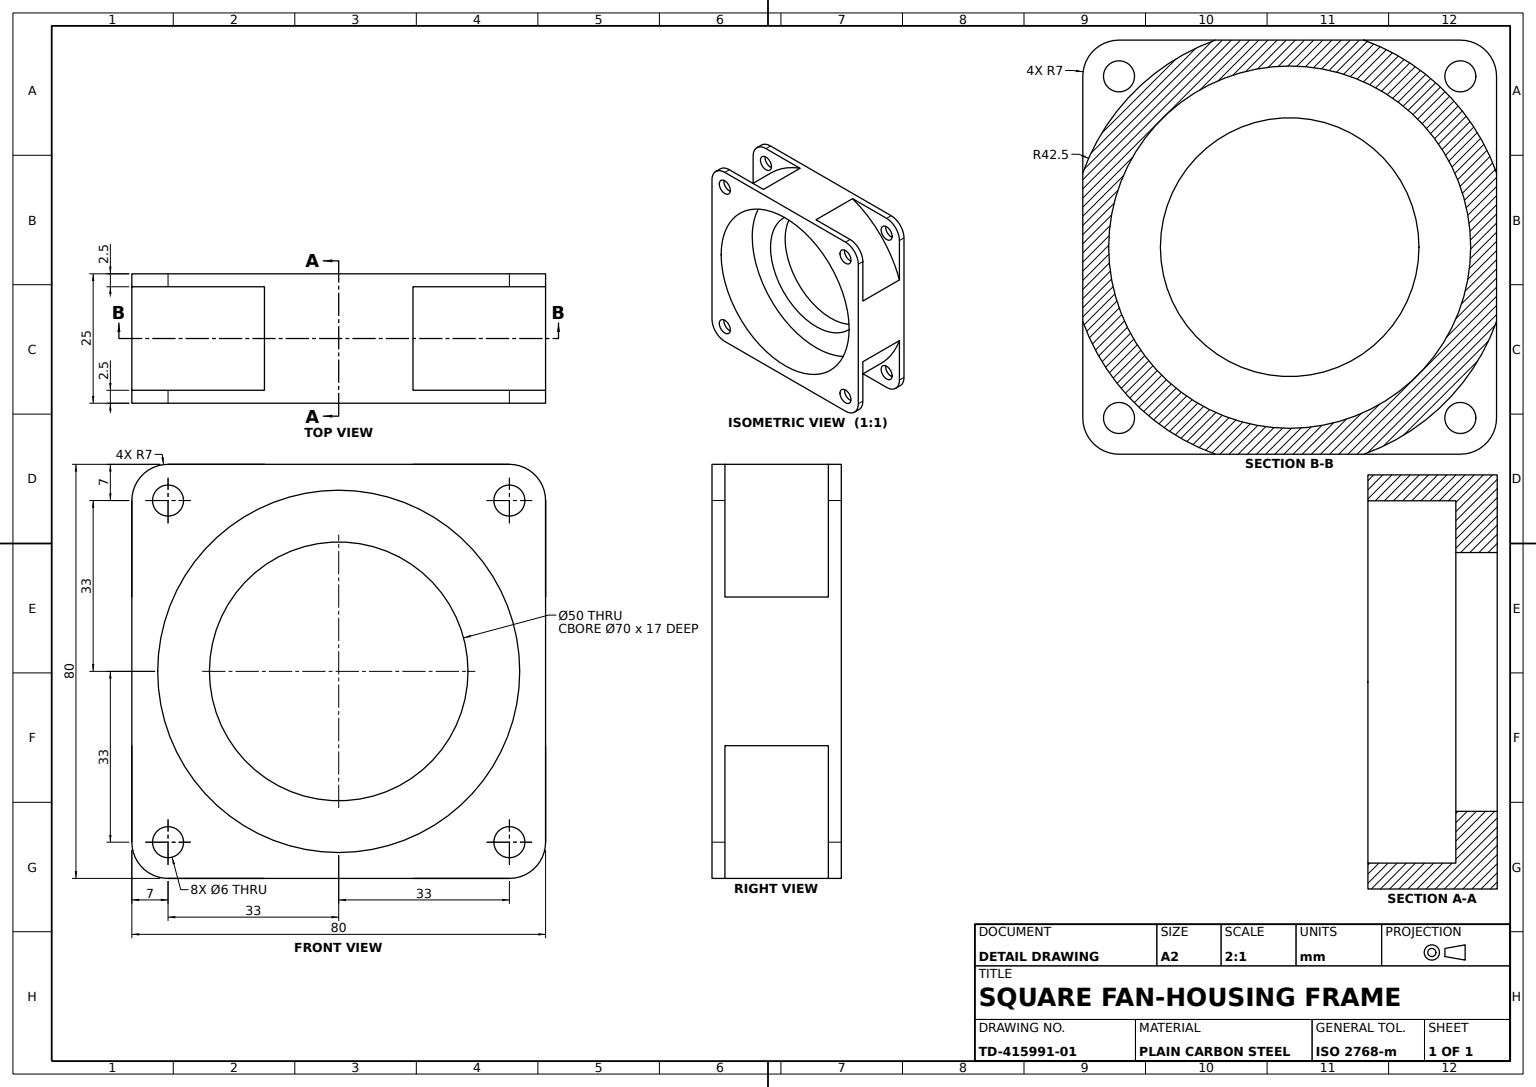
SolidWorks part; units mm, degrees
material "Plain Carbon Steel"
ref_plane "Front Plane" through (0, 0, 0) normal (0, 0, 1) x (1, 0, 0)
ref_plane "Top Plane" through (0, 0, 0) normal (0, 1, 0) x (1, 0, 0)
ref_plane "Right Plane" through (0, 0, 0) normal (1, 0, 0) x (0, 0, -1)
sketch "Front Flange Sketch" plane through (0, 0, 0) normal (0, 0, 1) x (1, 0, 0)
  line L1 (-33, -40) -> (33, -40)
  line L2 (-40, -33) -> (-40, 33)
  line L3 (-33, 40) -> (33, 40)
  line L4 (40, -33) -> (40, 33)
  line L5 (-40, -40) -> (40, 40) construction
  line L6 (-40, 40) -> (40, -40) construction
  arc A0 (33, 40) -> (40, 33) centre (33, 33) cw
  arc A1 (-33, -40) -> (-40, -33) centre (-33, -33) cw
  arc A2 (40, -33) -> (33, -40) centre (33, -33) cw
  arc A3 (-40, 33) -> (-33, 40) centre (-33, 33) cw
  point P0 (0, 0)
  dimension "D3" = 7
  dimension "D1" = 80
  dimension "D2" = 80
extrude "Front Flange 80x80" add sketch "Front Flange Sketch" against normal blind 2.5
sketch "Housing Body Sketch" plane through (0, 0, -2.5) normal (0, 0, -1) x (-1, 0, 0)
  line L0 (-14.3614, 40) -> (14.3614, 40)
  line L1 (-40, -33) -> (-40, 33) construction
  line L2 (40, 14.3614) -> (40, -14.3614)
  line L4 (14.3614, -40) -> (-14.3614, -40)
  line L6 (-40, 14.3614) -> (-40, -14.3614)
  arc A0 (-14.3614, 40) -> (-40, 14.3614) centre (0, 0) ccw
  arc A1 (40, 14.3614) -> (14.3614, 40) centre (0, 0) ccw
  arc A2 (14.3614, -40) -> (40, -14.3614) centre (0, 0) ccw
  arc A3 (-40, -14.3614) -> (-14.3614, -40) centre (0, 0) ccw
  dimension "D1" = 85
  dimension "D2" = 25.6386
extrude "Housing Body" add sketch "Housing Body Sketch" along normal blind 20
sketch "Rear Flange Sketch" plane through (0, 0, -22.5) normal (0, 0, -1) x (-1, 0, 0)
  line L1 (33, -40) -> (-33, -40)
  line L2 (40, -33) -> (40, 33)
  line L3 (33, 40) -> (-33, 40)
  line L4 (-40, -33) -> (-40, 33)
  line L5 (40, -40) -> (-40, 40) construction
  line L6 (40, 40) -> (-40, -40) construction
  arc A0 (-40, -33) -> (-33, -40) centre (-33, -33) ccw
  arc A1 (40, -33) -> (33, -40) centre (33, -33) cw
  arc A2 (40, 33) -> (33, 40) centre (33, 33) ccw
  arc A3 (-40, 33) -> (-33, 40) centre (-33, 33) cw
  point P0 (0, 0)
  dimension "D3" = 7
  dimension "D1" = 80
  dimension "D2" = 80
extrude "Rear Flange 80x80" add sketch "Rear Flange Sketch" along normal blind 2.5
sketch "Mounting Holes Sketch" plane through (0, 0, 0) normal (0, 0, 1) x (1, 0, 0)
  circle A0 centre (-33, 33) radius 3
  circle A1 centre (33, 33) radius 3
  circle A2 centre (33, -33) radius 3
  circle A3 centre (-33, -33) radius 3
  dimension "D1" = 6
  dimension "D2" = 6
  dimension "D3" = 6
  dimension "D4" = 6
extrude "Mounting Holes 4x" cut sketch "Mounting Holes Sketch" against normal blind 92.5
sketch "Through Bore Sketch Ø50" plane through (0, 0, 0) normal (0, 0, 1) x (1, 0, 0)
  circle A0 centre (0, 0) radius 25
  dimension "D1" = 50
extrude "Through Bore Ø50" cut sketch "Through Bore Sketch Ø50" against normal blind 132.5
sketch "Counterbore Sketch Ø70" plane through (0, 0, 0) normal (0, 0, 1) x (1, 0, 0)
  circle A0 centre (0, 0) radius 35
  dimension "D1" = 70
extrude "Counterbore Ø70" cut sketch "Counterbore Sketch Ø70" against normal blind 17
